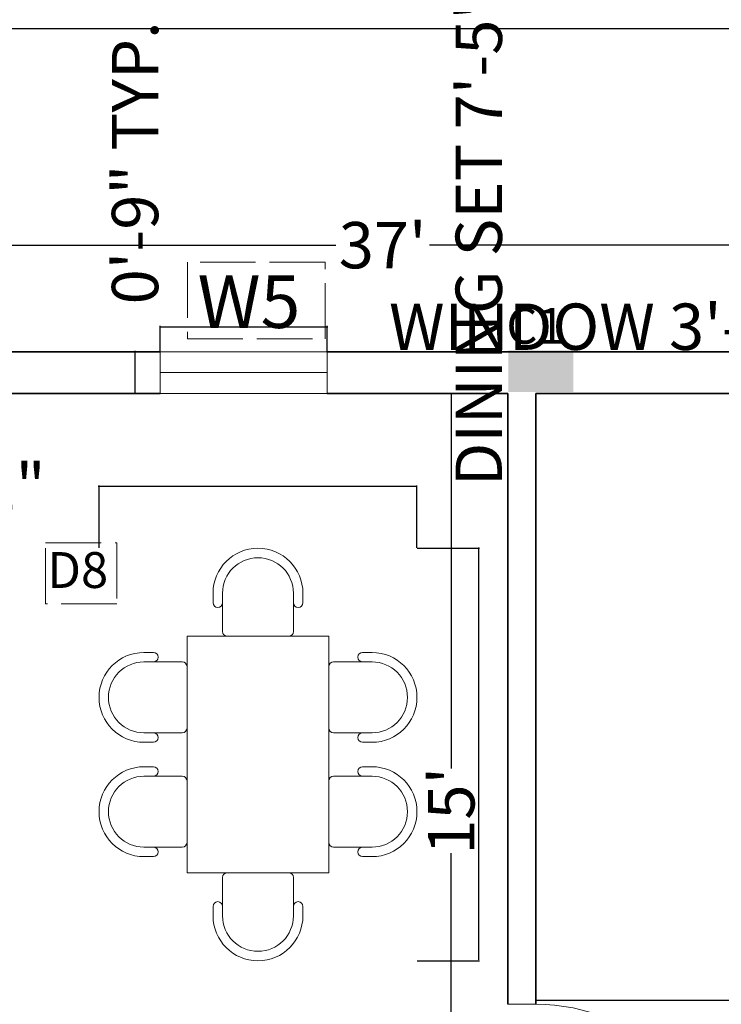
# Model space of a CAD drawing. Units: inches. Extents: x -269 to 4574, y -694 to 313.
# Tile 10 of 19: x 151 to 302, y -122 to 90. Entities that reach past the tile are written whole.
import ezdxf

# ---------------------------------------------------------------- set-up
doc = ezdxf.new("R2010")
doc.units = ezdxf.units.IN
doc.header["$MEASUREMENT"] = 0
doc.linetypes.add('ACAD_ISO02W100', pattern=[15, 12, -3])
for name, color, linetype, lineweight in [('A-ANNO-FRAM', 7, 'ACAD_ISO02W100', 13), ('A-ANNO-IDEN', 6, 'Continuous', 18), ('A-COLS', 5, 'Continuous', 35), ('A-COLS-IDEN', 6, 'Continuous', 18), ('A-FURN', 2, 'Continuous', 18), ('C-PROP', 7, 'Continuous', 25), ('DIMENSION', 5, 'Continuous', 18), ('DOORS', 3, 'Continuous', 18), ('WALL', 1, 'Continuous', 35), ('WINDOWS', 2, 'Continuous', 18)]:
    doc.layers.add(name, color=color, linetype=linetype, lineweight=lineweight)
doc.dimstyles.get("Standard").update_dxf_attribs({"dimtxt": 10, "dimasz": 0.18, "dimexe": 0.18, "dimexo": 0.0625, "dimgap": 0.09, "dimtad": 0, "dimdec": 1, "dimzin": 0, "dimdsep": 46, "dimlunit": 3, "dimtxsty": 'Standard', "dimcen": 0.09, "dimclrt": 7, "dimadec": 0, "dimazin": 0, "dimtfac": 1, "dimtdec": 1, "dimtofl": 0, "dimtmove": 0, "dimatfit": 3, "dimfxl": 1, "dimtolj": 1, "dimtzin": 0, "dimarcsym": 0})

# ---------------------------------------------------------------- blocks, each defined once
blk = doc.blocks.new('*D1')
at = {"layer": 'Defpoints', "color": 0, "lineweight": 0, "transparency": 16777216}
for p in [(451.14, 41.26), (7.14, 18.27), (451.14, 18.27)]:
    blk.add_point(p, dxfattribs=at)
at = {"layer": 'DIMENSION', "color": 0, "lineweight": -2, "transparency": 16777216}
for p, q in [((7.14, 18.33), (7.14, 41.44)), ((7.32, 41.26), (219.05, 41.26)), ((450.96, 41.26), (239.23, 41.26)), ((451.14, 18.33), (451.14, 41.44))]:
    blk.add_line(p, q, dxfattribs=at)
at = {"layer": 'DIMENSION', "color": 0, "lineweight": 0, "transparency": 16777216}
for points in [[(7.32, 41.29), (7.32, 41.23), (7.14, 41.26)], [(450.96, 41.29), (450.96, 41.23), (451.14, 41.26)]]:
    blk.add_solid(points, dxfattribs=at)
at = {"layer": 'DIMENSION', "color": 0, "transparency": 16777216, "insert": (229.14, 41.26), "char_height": 10, "attachment_point": 5}
blk.add_mtext("\\A1;37'", dxfattribs=at)
blk = doc.blocks.new('*U3')
for p, q in [((0, 0), (0, -6)), ((40, 0), (40, -6))]:
    blk.add_line(p, q)
blk.add_lwpolyline([(0, 0), (0, 40), (1.75, 40), (1.75, 0)], close=True)
blk.add_arc((0, 0), 40, 0, 90)
blk = doc.blocks.new('A$C5AA626B0')
for p, q in [((660.7, 1671.6), (660.7, 1731.6)), ((720.7, 1488.3), (720.7, 1731.6)), ((1170.7, 1731.6), (1170.7, 1488.3)), ((1230.7, 1731.6), (1230.7, 1671.6)), ((1385.9, 1731.6), (1385.9, 1671.6)), ((1445.9, 1731.6), (1445.9, 1488.3)), ((1895.9, 1488.3), (1895.9, 1731.6)), ((1955.9, 1671.6), (1955.9, 1731.6)), ((558.3, 1458.3), (2058.3, 1458.3)), ((558.3, 558.3), (558.3, 1458.3)), ((1475.9, 1458.3), (1865.9, 1458.3)), ((2058.3, 1458.3), (2058.3, 558.3)), ((285, 1293.3), (345, 1293.3)), ((2271.6, 1293.3), (2331.6, 1293.3)), ((285, 1233.3), (528.3, 1233.3)), ((558.3, 1203.3), (558.3, 813.3)), ((2058.3, 813.3), (2058.3, 1203.3)), ((2088.3, 1233.3), (2331.6, 1233.3)), ((528.3, 783.3), (285, 783.3)), ((2331.6, 783.3), (2088.3, 783.3)), ((345, 723.3), (285, 723.3)), ((2331.6, 723.3), (2271.6, 723.3)), ((2058.3, 558.3), (558.3, 558.3)), ((720.7, 528.3), (720.7, 285)), ((1170.7, 285), (1170.7, 528.3)), ((1445.9, 285), (1445.9, 528.3)), ((1475.9, 558.3), (1865.9, 558.3)), ((1895.9, 528.3), (1895.9, 285)), ((660.7, 345), (660.7, 285)), ((1230.7, 285), (1230.7, 345)), ((1385.9, 285), (1385.9, 345)), ((1955.9, 345), (1955.9, 285))]:
    blk.add_line(p, q)
for centre, radius, start, end in [((945.7, 1731.6), 285, 0, 180), ((1670.9, 1731.6), 285, 0, 180), ((945.7, 1731.6), 225, 0, 180), ((1670.9, 1731.6), 225, 0, 180), ((690.7, 1671.6), 30, 180, 0), ((1200.7, 1671.6), 30, 180, 0), ((1415.9, 1671.6), 30, 180, 0), ((1925.9, 1671.6), 30, 180, 0), ((750.7, 1488.3), 30, 180, 270), ((1140.7, 1488.3), 30, 270, 0), ((1475.9, 1488.3), 30, 180, 270), ((1865.9, 1488.3), 30, 270, 0), ((285, 1008.3), 285, 90, 270), ((345, 1263.3), 30, 270, 90), ((2271.6, 1263.3), 30, 90, 270), ((2331.6, 1008.3), 285, 270, 90), ((285, 1008.3), 225, 90, 270), ((528.3, 1203.3), 30, 0, 90), ((2088.3, 1203.3), 30, 90, 180), ((2331.6, 1008.3), 225, 270, 90), ((528.3, 813.3), 30, 270, 0), ((2088.3, 813.3), 30, 180, 270), ((345, 753.3), 30, 270, 90), ((2271.6, 753.3), 30, 90, 270), ((750.7, 528.3), 30, 90, 180), ((1140.7, 528.3), 30, 0, 90), ((1475.9, 528.3), 30, 90, 180), ((1865.9, 528.3), 30, 0, 90), ((690.7, 345), 30, 0, 180), ((1200.7, 345), 30, 0, 180), ((1415.9, 345), 30, 0, 180), ((1925.9, 345), 30, 0, 180), ((945.7, 285), 285, 180, 0), ((945.7, 285), 225, 180, 0), ((1670.9, 285), 285, 180, 0), ((1670.9, 285), 225, 180, 0)]:
    blk.add_arc(centre, radius, start, end)
blk = doc.blocks.new('*D18')
at = {"layer": 'Defpoints', "color": 0, "lineweight": 0, "transparency": 16777216}
for p in [(256.14, 9.27), (243.94, -170.73), (262.14, -170.73)]:
    blk.add_point(p, dxfattribs=at)
at = {"layer": 'DIMENSION', "color": 0, "lineweight": -2, "transparency": 16777216}
for p, q in [((256.07, 9.27), (243.76, 9.27)), ((243.94, 9.09), (243.94, -71.59)), ((243.94, -170.55), (243.94, -89.87)), ((262.07, -170.73), (243.76, -170.73))]:
    blk.add_line(p, q, dxfattribs=at)
at = {"layer": 'DIMENSION', "color": 0, "lineweight": 0, "transparency": 16777216}
for points in [[(243.91, 9.09), (243.97, 9.09), (243.94, 9.27)], [(243.91, -170.55), (243.97, -170.55), (243.94, -170.73)]]:
    blk.add_solid(points, dxfattribs=at)
at = {"layer": 'DIMENSION', "color": 0, "transparency": 16777216, "insert": (243.94, -80.73), "char_height": 10, "attachment_point": 5, "rotation": 90}
blk.add_mtext("\\A1;15'", dxfattribs=at)
blk = doc.blocks.new('*D20')
at = {"layer": 'Defpoints', "color": 0, "lineweight": 0, "transparency": 16777216}
for p in [(262.14, -122.44), (442.14, -121.56), (442.14, -122.44)]:
    blk.add_point(p, dxfattribs=at)
at = {"layer": 'DIMENSION', "color": 0, "lineweight": -2, "transparency": 16777216}
for p, q in [((262.14, -122.38), (262.14, -121.38)), ((262.32, -121.56), (343, -121.56)), ((441.96, -121.56), (361.27, -121.56)), ((442.14, -122.38), (442.14, -121.38))]:
    blk.add_line(p, q, dxfattribs=at)
at = {"layer": 'DIMENSION', "color": 0, "lineweight": 0, "transparency": 16777216}
for points in [[(262.32, -121.53), (262.32, -121.59), (262.14, -121.56)], [(441.96, -121.53), (441.96, -121.59), (442.14, -121.56)]]:
    blk.add_solid(points, dxfattribs=at)
at = {"layer": 'DIMENSION', "color": 0, "transparency": 16777216, "insert": (352.14, -121.56), "char_height": 10, "attachment_point": 5}
blk.add_mtext("\\A1;15'", dxfattribs=at)
blk = doc.blocks.new('GLAZ-36IN')
blk.add_line((0, 4.5), (36, 4.5))
blk.add_lwpolyline([(0, 9), (36, 9), (36, 0), (0, 0)], close=True)
blk = doc.blocks.new('TAG-DOOR-FRAME')
blk.add_lwpolyline([(0, 13.18), (15.39, 13.18), (15.39, 0), (0, 0)], close=True)
blk = doc.blocks.new('COLUMN-9x14-PLAN')
h = blk.add_hatch(color=256)
h.dxf.hatch_style = 1
h.paths.add_polyline_path([(9, 14), (0, 14), (0, 0), (9, 0), (9, 5)])
blk = doc.blocks.new('*D55')
at = {"layer": 'Defpoints', "color": 0, "lineweight": 0, "transparency": 16777216}
for p in [(217.14, 23.67), (181.14, 18.27), (217.14, 18.27)]:
    blk.add_point(p, dxfattribs=at)
at = {"layer": 'DIMENSION', "color": 0, "lineweight": -2, "transparency": 16777216}
for p, q in [((181.14, 18.33), (181.14, 23.85)), ((181.32, 23.67), (216.96, 23.67)), ((217.14, 18.33), (217.14, 23.85)), ((217.14, 23.67), (217.32, 23.67))]:
    blk.add_line(p, q, dxfattribs=at)
at = {"layer": 'DIMENSION', "color": 0, "lineweight": 0, "transparency": 16777216}
for points in [[(181.32, 23.7), (181.32, 23.64), (181.14, 23.67)], [(216.96, 23.7), (216.96, 23.64), (217.14, 23.67)]]:
    blk.add_solid(points, dxfattribs=at)
at = {"layer": 'DIMENSION', "color": 7, "transparency": 16777216, "insert": (291.22, 23.67), "char_height": 10, "attachment_point": 5}
blk.add_mtext('\\A1;WINDOW 3\'-0" TYP.', dxfattribs=at)
blk = doc.blocks.new('*D56')
at = {"layer": 'Defpoints', "color": 0, "lineweight": 0, "transparency": 16777216}
for p in [(175.74, 18.27), (181.14, 18.27), (181.14, 9.27)]:
    blk.add_point(p, dxfattribs=at)
at = {"layer": 'DIMENSION', "color": 0, "lineweight": -2, "transparency": 16777216}
for p, q in [((181.07, 18.27), (175.56, 18.27)), ((175.74, 18.27), (175.74, 18.45)), ((175.74, 9.45), (175.74, 18.09)), ((181.07, 9.27), (175.56, 9.27))]:
    blk.add_line(p, q, dxfattribs=at)
at = {"layer": 'DIMENSION', "color": 0, "lineweight": 0, "transparency": 16777216}
for points in [[(175.71, 18.09), (175.77, 18.09), (175.74, 18.27)], [(175.71, 9.45), (175.77, 9.45), (175.74, 9.27)]]:
    blk.add_solid(points, dxfattribs=at)
at = {"layer": 'DIMENSION', "color": 7, "transparency": 16777216, "insert": (175.74, 59.01), "char_height": 10, "attachment_point": 5, "rotation": 90}
blk.add_mtext('\\A1;0\'-9" TYP.', dxfattribs=at)
blk = doc.blocks.new('*D65')
at = {"layer": 'Defpoints', "color": 0, "lineweight": 0, "transparency": 16777216}
for p in [(236.53, -24.12), (249.87, -24.12), (236.53, -113.07)]:
    blk.add_point(p, dxfattribs=at)
at = {"layer": 'DIMENSION', "color": 0, "lineweight": -2, "transparency": 16777216}
for p, q in [((236.59, -24.12), (250.05, -24.12)), ((249.87, -24.12), (249.87, -23.94)), ((249.87, -112.89), (249.87, -24.3)), ((236.59, -113.07), (250.05, -113.07))]:
    blk.add_line(p, q, dxfattribs=at)
at = {"layer": 'DIMENSION', "color": 0, "lineweight": 0, "transparency": 16777216}
for points in [[(249.84, -24.3), (249.9, -24.3), (249.87, -24.12)], [(249.84, -112.89), (249.9, -112.89), (249.87, -113.07)]]:
    blk.add_solid(points, dxfattribs=at)
at = {"layer": 'DIMENSION', "color": 7, "transparency": 16777216, "insert": (249.87, 42.82), "char_height": 10, "attachment_point": 5, "rotation": 90}
blk.add_mtext('\\A1;DINING SET 7\'-5"', dxfattribs=at)
blk = doc.blocks.new('*D66')
at = {"layer": 'Defpoints', "color": 0, "lineweight": 0, "transparency": 16777216}
for p in [(167.97, -10.77), (167.97, -24.12), (236.53, -24.12)]:
    blk.add_point(p, dxfattribs=at)
at = {"layer": 'DIMENSION', "color": 0, "lineweight": -2, "transparency": 16777216}
for p, q in [((167.97, -24.05), (167.97, -10.59)), ((236.53, -24.05), (236.53, -10.59)), ((167.97, -10.77), (167.79, -10.77)), ((236.35, -10.77), (168.15, -10.77))]:
    blk.add_line(p, q, dxfattribs=at)
at = {"layer": 'DIMENSION', "color": 0, "lineweight": 0, "transparency": 16777216}
for points in [[(168.15, -10.74), (168.15, -10.8), (167.97, -10.77)], [(236.35, -10.74), (236.35, -10.8), (236.53, -10.77)]]:
    blk.add_solid(points, dxfattribs=at)
at = {"layer": 'DIMENSION', "color": 7, "transparency": 16777216, "insert": (129.6, -10.77), "char_height": 10, "attachment_point": 5}
blk.add_mtext('\\A1;5\'-8 1/2"', dxfattribs=at)

msp = doc.modelspace()

# ---------------------------------------------------------------- linework, layer by layer
at = {"layer": 'A-ANNO-FRAM'}
msp.add_lwpolyline([(216.75, 37.56), (187.02, 37.56), (187.02, 21.05), (216.75, 21.05)], close=True, dxfattribs=at)
at = {"layer": 'C-PROP'}
msp.add_line((-37.71, 88), (478.29, 88), dxfattribs=at)
at = {"layer": 'WALL'}
for p, q in [((94.14, 18.27), (181.14, 18.27)), ((217.14, 18.27), (332.64, 18.27)), ((142.14, 9.27), (181.14, 9.27)), ((217.14, 9.27), (256.14, 9.27)), ((256.14, -122.44), (256.14, 9.27)), ((262.14, 9.27), (332.64, 9.27)), ((262.14, -122.44), (262.14, 9.27))]:
    msp.add_line(p, q, dxfattribs=at)

# ---------------------------------------------------------------- block references
at = {"layer": 'A-ANNO-FRAM', "rotation": 180}
msp.add_blockref('TAG-DOOR-FRAME', (171.83, -22.94), dxfattribs=at)
at = {"layer": 'A-COLS', "rotation": 89.99999999999984}
msp.add_blockref('COLUMN-9x14-PLAN', (270.26, 9.6), dxfattribs=at)
at = {"layer": 'A-FURN', "xscale": 0.0339971369196016, "yscale": 0.0339971369196016, "zscale": 0.0339971369196016, "rotation": 90}
msp.add_blockref('A$C5AA626B0', (236.53, -113.07), dxfattribs=at)
at = {"layer": 'DOORS', "xscale": -1, "rotation": 270}
msp.add_blockref('*U3', (262.14, -162.44), dxfattribs=at)
at = {"layer": 'WINDOWS'}
msp.add_blockref('GLAZ-36IN', (181.14, 9.27), dxfattribs=at)

# ---------------------------------------------------------------- texts
at = {"layer": 'A-ANNO-IDEN'}
for s, height, p in [('W5', 11.343, (189.22, 23.4)), ('D8', 7.741, (156.82, -32.67))]:
    msp.add_text(s, height=height, dxfattribs=at).set_placement(p)
at = {"layer": 'A-COLS-IDEN'}
msp.add_text('C1', height=7.741, dxfattribs=at).set_placement((255.8, 19.99))

# ---------------------------------------------------------------- dimensions: what is measured, and where the dimension line sits
at = {"layer": 'DIMENSION'}
for base, p1, p2, text, picture, middle in [((249.8693, -24.1158), (236.5257, -113.0737), (236.5257, -24.1158), 'DINING SET <>', '*D65', (249.8693, 42.8209)), ((175.74, 18.27), (181.14, 9.27), (181.14, 18.27), '<> TYP.', '*D56', (175.74, 59.01))]:
    dim = msp.add_linear_dim(base=base, p1=p1, p2=p2, angle=90, text=text, dimstyle='Standard', override={"dimdec": 1, "dimlfac": 1, "dimrnd": 0, "dimzin": 1, "dimdsep": 46, "dimlunit": 4, "dimfrac": 2}, dxfattribs=at)
    dim.commit()
    dim.dimension.update_dxf_attribs({"geometry": picture, "text_midpoint": middle})
for base, p1, p2, picture, middle in [((451.14, 41.26), (7.14, 18.27), (451.14, 18.27), '*D1', (229.14, 41.26)), ((442.14, -121.56), (262.14, -122.44), (442.14, -122.44), '*D20', (352.14, -121.56))]:
    dim = msp.add_linear_dim(base=base, p1=p1, p2=p2, dimstyle='Standard', override={"dimclrd": 0, "dimclre": 0, "dimclrt": 0}, dxfattribs=at)
    dim.commit()
    dim.dimension.update_dxf_attribs({"geometry": picture, "text_midpoint": middle})
dim = msp.add_linear_dim(base=(217.14, 23.67), p1=(181.14, 18.27), p2=(217.14, 18.27), text='WINDOW <> TYP.', dimstyle='Standard', override={"dimdec": 1, "dimlfac": 1, "dimrnd": 0, "dimzin": 1, "dimdsep": 46, "dimlunit": 4, "dimfrac": 2}, dxfattribs=at)
dim.commit()
dim.dimension.update_dxf_attribs({"geometry": '*D55', "text_midpoint": (291.22, 23.67)})
for base, p1, p2, angle, override, picture, middle in [((243.94, -170.73), (256.14, 9.27), (262.14, -170.73), 90, {"dimclrd": 0, "dimclre": 0, "dimclrt": 0}, '*D18', (243.94, -80.73)), ((167.97, -10.77), (236.53, -24.12), (167.97, -24.12), 180, {"dimdec": 1, "dimlfac": 1, "dimrnd": 0, "dimzin": 1, "dimdsep": 46, "dimlunit": 4, "dimfrac": 2}, '*D66', (129.6, -10.77))]:
    dim = msp.add_linear_dim(base=base, p1=p1, p2=p2, angle=angle, dimstyle='Standard', override=override, dxfattribs=at)
    dim.commit()
    dim.dimension.update_dxf_attribs({"geometry": picture, "text_midpoint": middle})

doc.saveas('drawing.dxf')
